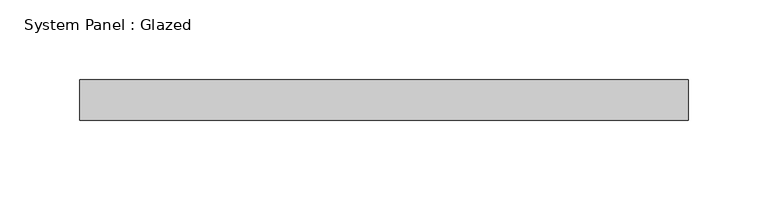
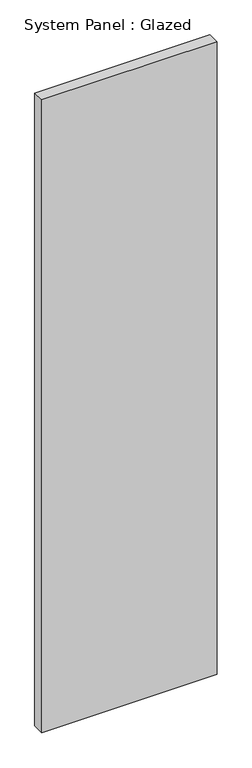
"""IFC4 building model written with IfcOpenShell, lengths in millimetres: plate geometry, System Panel : Glazed."""

from ifc_helpers import new_model, si_unit, origin, origin_with_axes, place, context, project, spatial, polyline, outline, extrude, source, transform, mapped, element, save


def system_panel_glazed_232e26bf(model_context):
    return source(origin(), model_context, "Body", "SweptSolid", [
        extrude(outline(polyline([(190.5, 19.05), (-190.5, 19.05), (-190.5, 44.45), (190.5, 44.45), (190.5, 19.05)])), origin_with_axes(), (0.0, 0.0, 1.0), 1453.0534505),
    ])


if __name__ == "__main__":
    model = new_model("IFC4")
    model_context = context("Model", 3, world=origin())
    ifc_project = project(units=[si_unit("LENGTHUNIT", "METRE", prefix="MILLI")], contexts=[model_context])
    site = spatial("IfcSite", under=ifc_project)
    building = spatial("IfcBuilding", under=site)
    placement = place(None, origin())
    system_panel_glazed_shape = system_panel_glazed_232e26bf(model_context)
    element("IfcPlate", 1, ObjectType="System Panel : Glazed", at=placement, inside=building, context=model_context, shape_type="MappedRepresentation", body=[
        mapped(system_panel_glazed_shape, transform((0.0, 0.0, 0.0), x_axis=(1.0, 0.0, 0.0), y_axis=(0.0, 1.0, 0.0), z_axis=(0.0, 0.0, 1.0))),
    ])
    save(model, "model.ifc")

# Revit data of these elements
# Type "System Panel : Glazed"
#   Construction Type Id = "GSP4R"
#   Analytic Construction = "1/8 in Pilkington single glazing"
#   Visual Light Transmittance = 0.9
#   Solar Heat Gain Coefficient = 0.86
#   Heat Transfer Coefficient (U) = 1.18115 BTU/(h·ft²·°F)
#   Define Thermal Properties by = 1
# Element 1 (IfcPlate, "System Panel : Glazed")
#   Materials on its faces: "Glass"
# Materials
#   "Glass": class "Glass", colour RGB 0 128 192, transparency 0.75, Description = "Soda Lime Glass", Cost = 0
